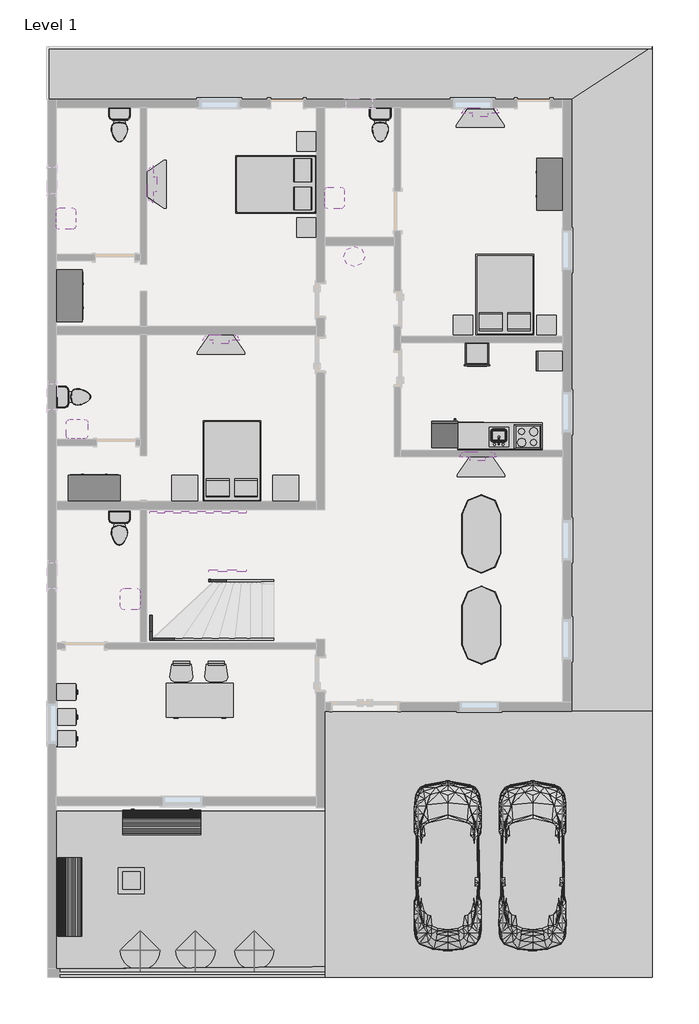
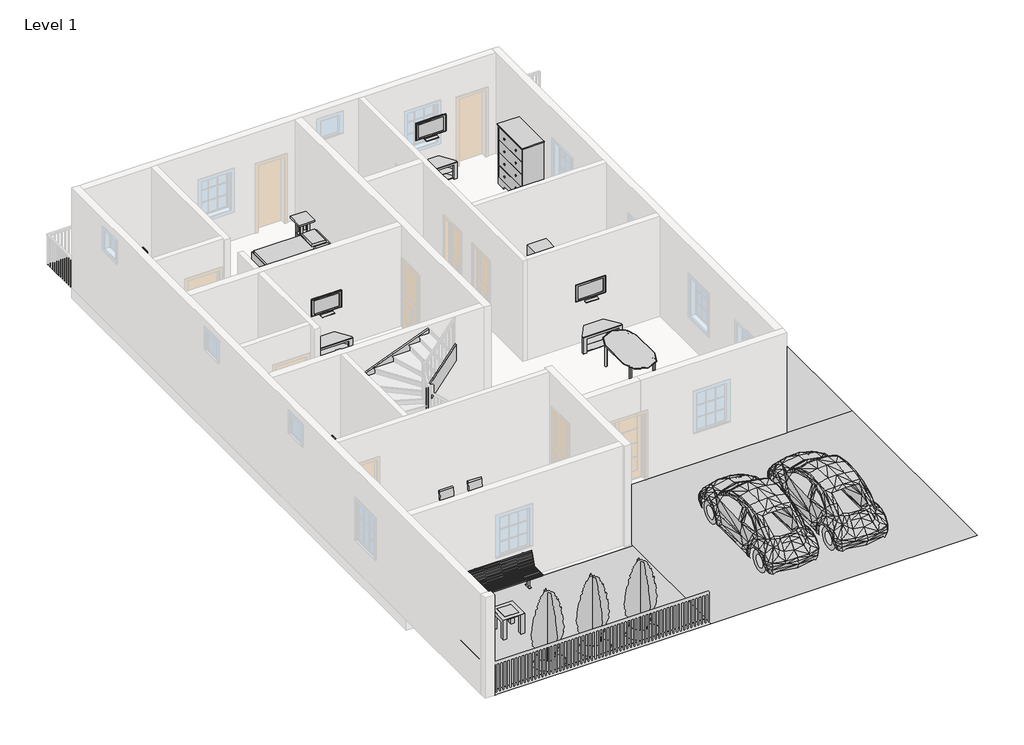
# One storey, part 4 of 4: 30 furniture elements, 13 proxies, 10 flow terminals, 8 members, 5 geographic elements.
"""IFC4 building model written with IfcOpenShell, lengths in millimetres."""

from ifc_helpers import new_model, si_unit, frame, origin, place, context, project, spatial, polyline, outline, extrude, triangles, transform, mapped, element, save
from components import proxy_7e1014cc, proxy_a6faaae8, proxy_45b28599, kitchenette_medium_kitchenette_medium_844211aa, proxy_8b8c2dc4, rpc_beetle_rpc_beetle_3ce7ba48, proxy_c523a7b7, flow_terminal_871c2e40, flow_terminal_d49f872f, flow_terminal_62a433f7, toilet_domestic_3d_toilet_domestic_3d_f7549cf7, toilet_domestic_3d_toilet_domestic_3d_183bbd19, furniture_c8abb964, furniture_bb55ed6b, chair_desk_chair_desk_ccc35c8f, furniture_c6510c7c, furniture_013ab306, furniture_9fa109b2, furniture_56245f3a, tv_stand_tv_stand_6ce107e5, furniture_b5c51a22, furniture_2c34a4f9, furniture_097b63cf, furniture_5bc9ed15, geographic_element_235d1464, rpc_tree_conifer_0001_chinese_juniper_7_1b9786cd

model = new_model("IFC4")

# Units and contexts
model_context = context("Model", 3, world=origin())
ifc_project = project(units=[si_unit("LENGTHUNIT", "METRE", prefix="MILLI")], contexts=[model_context])

# Site, building, storey
site = spatial("IfcSite", under=ifc_project)
building = spatial("IfcBuilding", under=site)
storey = spatial("IfcBuildingStorey", under=building, Name="Level 1", Elevation=0.0)

# Proxies
placement = place(None, origin())
element("IfcBuildingElementProxy", 1, Name="Building Element Proxy", at=placement, inside=storey, context=model_context, shape_type="Tessellation", body=[
    triangles([(-5541.2013062, 9210.7988297, 0.0), (-5541.2013062, 10429.9982483, 0.0), (8581.1988876, 10429.9982483, 0.0), (6701.5985001, 9210.7988297, 0.0)], [[2, 1, 4], [4, 3, 2]], closed=False),
])
element("IfcBuildingElementProxy", 2, Name="Building Element Proxy", at=placement, inside=storey, context=model_context, shape_type="Tessellation", body=[
    triangles([(6701.5985001, 9210.7988297, 0.0), (8581.1988876, 10429.9982483, 0.0), (6701.5985001, -5089.4009766, 0.0), (8581.1988876, -5089.4009766, 0.0)], [[1, 3, 4], [4, 2, 1]], closed=False),
])
element("IfcBuildingElementProxy", 3, Name="Building Element Proxy", at=placement, inside=storey, context=model_context, shape_type="Tessellation", body=[
    triangles([(935.7986212, -11312.4013641, 0.0), (935.7986212, -7350.0013641, 0.0), (935.7986212, -5089.4009766, 0.0), (8581.1988876, -5089.4009766, 0.0), (8581.1988876, -11312.4013641, 0.0)], [[2, 4, 3], [2, 5, 4], [5, 2, 1]], closed=False),
])
element("IfcBuildingElementProxy", 4, Name="Building Element Proxy", at=placement, inside=storey, context=model_context, shape_type="Tessellation", body=[
    triangles([(-5338.0014999, -11109.2009766, 0.0), (-5329.5107391, -7423.5707108, 0.0), (934.8501326, -7422.4108978, 0.0), (935.7986212, -11058.4017517, 0.0)], [[2, 1, 4], [4, 3, 2]], closed=False),
])
element("IfcBuildingElementProxy", 5, Name="Building Element Proxy", at=placement, inside=storey, context=model_context, shape_type="Tessellation", body=[
    triangles([(932.4697546, -11067.6383972, 0.0), (935.7986212, -11312.4013641, 0.0), (-5261.8014999, -11109.2009766, 0.0), (-5242.6887131, -11312.4013641, 0.0), (-5261.8014999, -11312.4013641, 0.0)], [[3, 5, 4], [4, 2, 1], [4, 1, 3]], closed=False),
])
proxy_shape = proxy_7e1014cc(model_context)
element("IfcBuildingElementProxy", 6, Name="18\" x 24\" x 34 1/2\"", ObjectType="18\" x 24\" x 34 1/2\"", at=placement, inside=storey, context=model_context, shape_type="MappedRepresentation", body=[
    mapped(proxy_shape, transform((5927.1490822, 3395.5162793, 0.0), x_axis=(0.0, -1.0000000000000009, 0.0), y_axis=(1.0000000000000009, 0.0, 0.0), z_axis=(0.0, 0.0, 1.0))),
])
proxy_2_shape = proxy_a6faaae8(model_context)
element("IfcBuildingElementProxy", 7, Name="Cook Top-4 Unit2 : 22\" x 20\"", ObjectType="Cook Top-4 Unit2 : 22\" x 20\"", at=placement, inside=storey, context=model_context, shape_type="MappedRepresentation", body=[
    mapped(proxy_2_shape, transform((5672.898647, 1311.3988108, 0.0), x_axis=(-1.0000000000000004, 0.0, 0.0), y_axis=(0.0, -1.0000000000000004, 0.0), z_axis=(0.0, 0.0, 1.0))),
])
proxy_3_shape = proxy_45b28599(model_context)
element("IfcBuildingElementProxy", 8, Name="Dishwasher : 24\" x 24\" x 34\"", ObjectType="Dishwasher : 24\" x 24\" x 34\"", at=placement, inside=storey, context=model_context, shape_type="MappedRepresentation", body=[
    mapped(proxy_3_shape, transform((4721.7161155, 1603.2483756, 0.0), x_axis=(-1.0000000000000004, 0.0, 0.0), y_axis=(0.0, -1.0000000000000004, 0.0), z_axis=(0.0, 0.0, 1.0))),
])
kitchenette_medium_kitchenette_medium_shape = kitchenette_medium_kitchenette_medium_844211aa(model_context)
element("IfcBuildingElementProxy", 9, Name="Kitchenette - Medium : Kitchenette - Medium", ObjectType="Kitchenette - Medium : Kitchenette - Medium", at=placement, inside=storey, context=model_context, shape_type="MappedRepresentation", body=[
    mapped(kitchenette_medium_kitchenette_medium_shape, transform((5348.7363519, 1006.5988108, 0.0), x_axis=(-1.0000000000000004, 0.0, 0.0), y_axis=(0.0, -1.0000000000000004, 0.0), z_axis=(0.0, 0.0, 1.0))),
])
proxy_4_shape = proxy_8b8c2dc4(model_context)
element("IfcBuildingElementProxy", 10, Name="Oven Double-Built-in : 21 1/2\" x 39 1/4\" x 21\"", ObjectType="Oven Double-Built-in : 21 1/2\" x 39 1/4\" x 21\"", at=placement, inside=storey, context=model_context, shape_type="MappedRepresentation", body=[
    mapped(proxy_4_shape, transform((4526.9735743, 3126.1329519, 0.0), x_axis=(1.0, 0.0, 0.0), y_axis=(0.0, 1.0, 0.0), z_axis=(0.0, 0.0, 1.0))),
])
rpc_beetle_rpc_beetle_shape = rpc_beetle_rpc_beetle_3ce7ba48(model_context)
element("IfcBuildingElementProxy", 11, Name="RPC Beetle : RPC Beetle", ObjectType="RPC Beetle : RPC Beetle", at=placement, inside=storey, context=model_context, shape_type="MappedRepresentation", body=[
    mapped(rpc_beetle_rpc_beetle_shape, transform((5787.198647, -9940.8011892, 0.0), x_axis=(1.0, 0.0, 0.0), y_axis=(0.0, 1.0, 0.0), z_axis=(0.0, 0.0, 1.0))),
])
element("IfcBuildingElementProxy", 12, Name="RPC Beetle : RPC Beetle", ObjectType="RPC Beetle : RPC Beetle", at=placement, inside=storey, context=model_context, shape_type="MappedRepresentation", body=[
    mapped(rpc_beetle_rpc_beetle_shape, transform((3805.998647, -9940.8011892, 0.0), x_axis=(1.0, 0.0, 0.0), y_axis=(0.0, 1.0, 0.0), z_axis=(0.0, 0.0, 1.0))),
])
proxy_5_shape = proxy_c523a7b7(model_context)
element("IfcBuildingElementProxy", 13, Name="Refrigerator : 24\" x 25\" LH", ObjectType="Refrigerator : 24\" x 25\" LH", at=placement, inside=storey, context=model_context, shape_type="MappedRepresentation", body=[
    mapped(proxy_5_shape, transform((3736.148647, 1357.0477823, 0.0), x_axis=(-1.0000000000000004, 0.0, 0.0), y_axis=(0.0, -1.0000000000000004, 0.0), z_axis=(0.0, 0.0, 1.0))),
])

# Flow terminals
flow_terminal_shape = flow_terminal_871c2e40(model_context)
element("IfcFlowTerminal", 14, ObjectType="Sink Kitchen-Island : 18\" x 18\"", at=placement, inside=storey, context=model_context, shape_type="MappedRepresentation", body=[
    mapped(flow_terminal_shape, transform((5015.4878876, 1313.7442119, -14.4), x_axis=(-1.0000000000000004, 0.0, 0.0), y_axis=(0.0, -1.0000000000000004, 0.0), z_axis=(0.0, 0.0, 1.0))),
])
flow_terminal_2_shape = flow_terminal_d49f872f(model_context)
element("IfcFlowTerminal", 15, ObjectType="Sink Vanity-Round : 19\" x 19\"", at=placement, inside=storey, context=model_context, shape_type="MappedRepresentation", body=[
    mapped(flow_terminal_2_shape, transform((1524.9469064, 5444.8120813, 914.4), x_axis=(1.0, 0.0, 0.0), y_axis=(0.0, 1.0, 0.0), z_axis=(0.0, 0.0, 1.0))),
])
flow_terminal_3_shape = flow_terminal_62a433f7(model_context)
element("IfcFlowTerminal", 16, ObjectType="Sink Vanity-Square : 20\" x 18\"", at=placement, inside=storey, context=model_context, shape_type="MappedRepresentation", body=[
    mapped(flow_terminal_3_shape, transform((-5157.8559519, 6401.1095702, 914.4), x_axis=(0.0, 1.0, 0.0), y_axis=(-1.0, 0.0, 0.0), z_axis=(0.0, 0.0, 1.0))),
])
element("IfcFlowTerminal", 17, ObjectType="Sink Vanity-Square : 20\" x 18\"", at=placement, inside=storey, context=model_context, shape_type="MappedRepresentation", body=[
    mapped(flow_terminal_3_shape, transform((1115.9440481, 6883.7095702, 914.4), x_axis=(0.0, 1.0000000000000002, 0.0), y_axis=(-1.0000000000000002, 0.0, 0.0), z_axis=(0.0, 0.0, 1.0))),
])
element("IfcFlowTerminal", 18, ObjectType="Sink Vanity-Square : 20\" x 18\"", at=placement, inside=storey, context=model_context, shape_type="MappedRepresentation", body=[
    mapped(flow_terminal_3_shape, transform((-4839.7121124, 1453.4442119, 914.4), x_axis=(-1.0, 0.0, 0.0), y_axis=(0.0, -1.0, 0.0), z_axis=(0.0, 0.0, 1.0))),
])
element("IfcFlowTerminal", 19, ObjectType="Sink Vanity-Square : 20\" x 18\"", at=placement, inside=storey, context=model_context, shape_type="MappedRepresentation", body=[
    mapped(flow_terminal_3_shape, transform((-3562.3467541, -2457.5119486, 914.4), x_axis=(0.0, -1.0000000000000004, 0.0), y_axis=(1.0000000000000004, 0.0, 0.0), z_axis=(0.0, 0.0, 1.0))),
])
toilet_domestic_3d_toilet_domestic_3d_shape = toilet_domestic_3d_toilet_domestic_3d_f7549cf7(model_context)
toilet_domestic_3d_toilet_domestic_3d_2_shape = toilet_domestic_3d_toilet_domestic_3d_183bbd19(model_context)
element("IfcFlowTerminal", 20, ObjectType="Toilet-Domestic-3D : Toilet-Domestic-3D", at=placement, inside=storey, context=model_context, shape_type="MappedRepresentation", body=[
    mapped(toilet_domestic_3d_toilet_domestic_3d_shape, transform((-4843.3053257, 2251.1988108, 0.0), x_axis=(0.0, 1.0000000000000002, 0.0), y_axis=(-1.0000000000000002, 0.0, 0.0), z_axis=(0.0, 0.0, 1.0))),
    mapped(toilet_domestic_3d_toilet_domestic_3d_2_shape, transform((-4843.3053257, 2251.1988108, 0.0), x_axis=(0.0, 1.0000000000000002, 0.0), y_axis=(-1.0000000000000002, 0.0, 0.0), z_axis=(0.0, 0.0, 1.0))),
])
element("IfcFlowTerminal", 21, ObjectType="Toilet-Domestic-3D : Toilet-Domestic-3D", at=placement, inside=storey, context=model_context, shape_type="MappedRepresentation", body=[
    mapped(toilet_domestic_3d_toilet_domestic_3d_shape, transform((-3864.801353, 8512.9027835, 0.0), x_axis=(1.0, 0.0, 0.0), y_axis=(0.0, 1.0, 0.0), z_axis=(0.0, 0.0, 1.0))),
    mapped(toilet_domestic_3d_toilet_domestic_3d_2_shape, transform((-3864.801353, 8512.9027835, 0.0), x_axis=(1.0, 0.0, 0.0), y_axis=(0.0, 1.0, 0.0), z_axis=(0.0, 0.0, 1.0))),
])
element("IfcFlowTerminal", 22, ObjectType="Toilet-Domestic-3D : Toilet-Domestic-3D", at=placement, inside=storey, context=model_context, shape_type="MappedRepresentation", body=[
    mapped(toilet_domestic_3d_toilet_domestic_3d_shape, transform((2231.198647, 8512.9027835, 0.0), x_axis=(1.0, 0.0, 0.0), y_axis=(0.0, 1.0, 0.0), z_axis=(0.0, 0.0, 1.0))),
    mapped(toilet_domestic_3d_toilet_domestic_3d_2_shape, transform((2231.198647, 8512.9027835, 0.0), x_axis=(1.0, 0.0, 0.0), y_axis=(0.0, 1.0, 0.0), z_axis=(0.0, 0.0, 1.0))),
])
element("IfcFlowTerminal", 23, ObjectType="Toilet-Domestic-3D : Toilet-Domestic-3D", at=placement, inside=storey, context=model_context, shape_type="MappedRepresentation", body=[
    mapped(toilet_domestic_3d_toilet_domestic_3d_shape, transform((-3864.801353, -910.4972165, 0.0), x_axis=(1.0, 0.0, 0.0), y_axis=(0.0, 1.0, 0.0), z_axis=(0.0, 0.0, 1.0))),
    mapped(toilet_domestic_3d_toilet_domestic_3d_2_shape, transform((-3864.801353, -910.4972165, 0.0), x_axis=(1.0, 0.0, 0.0), y_axis=(0.0, 1.0, 0.0), z_axis=(0.0, 0.0, 1.0))),
])

# Furniture
furniture_shape = furniture_c8abb964(model_context)
element("IfcFurniture", 24, ObjectType="Bed-Box : Double 53\" x 74\"", at=placement, inside=storey, context=model_context, shape_type="MappedRepresentation", body=[
    mapped(furniture_shape, transform((-896.748894, 518.1693026, 0.0), x_axis=(-1.0, 0.0, 0.0), y_axis=(0.0, -1.0, 0.0), z_axis=(0.0, 0.0, 1.0))),
])
element("IfcFurniture", 25, ObjectType="Bed-Box : Double 53\" x 74\"", at=placement, inside=storey, context=model_context, shape_type="MappedRepresentation", body=[
    mapped(furniture_shape, transform((27.2281552, 7556.0512698, 0.0), x_axis=(0.0, -1.0000000000000002, 0.0), y_axis=(1.0000000000000002, 0.0, 0.0), z_axis=(0.0, 0.0, 1.0))),
])
element("IfcFurniture", 26, ObjectType="Bed-Box : Double 53\" x 74\"", at=placement, inside=storey, context=model_context, shape_type="MappedRepresentation", body=[
    mapped(furniture_shape, transform((5478.651106, 4404.3693026, 0.0), x_axis=(-1.0, 0.0, 0.0), y_axis=(0.0, -1.0, 0.0), z_axis=(0.0, 0.0, 1.0))),
])
furniture_2_shape = furniture_bb55ed6b(model_context)
element("IfcFurniture", 27, ObjectType="Cabinet-File 2 Drawer : 15\" x 18\"", at=placement, inside=storey, context=model_context, shape_type="MappedRepresentation", body=[
    mapped(furniture_2_shape, transform((-5251.5356531, -5609.2047422, 0.0), x_axis=(0.0, 1.0000000000000002, 0.0), y_axis=(-1.0000000000000002, 0.0, 0.0), z_axis=(0.0, 0.0, 1.0))),
])
element("IfcFurniture", 28, ObjectType="Cabinet-File 2 Drawer : 15\" x 18\"", at=placement, inside=storey, context=model_context, shape_type="MappedRepresentation", body=[
    mapped(furniture_2_shape, transform((-5251.5356531, -5101.2047422, 0.0), x_axis=(0.0, 1.0000000000000002, 0.0), y_axis=(-1.0000000000000002, 0.0, 0.0), z_axis=(0.0, 0.0, 1.0))),
])
element("IfcFurniture", 29, ObjectType="Cabinet-File 2 Drawer : 15\" x 18\"", at=placement, inside=storey, context=model_context, shape_type="MappedRepresentation", body=[
    mapped(furniture_2_shape, transform((-5251.5356531, -4517.0047422, 0.0), x_axis=(0.0, 1.0000000000000002, 0.0), y_axis=(-1.0000000000000002, 0.0, 0.0), z_axis=(0.0, 0.0, 1.0))),
])
chair_desk_chair_desk_shape = chair_desk_chair_desk_ccc35c8f(model_context)
element("IfcFurniture", 30, ObjectType="Chair-Desk : Chair-Desk", at=placement, inside=storey, context=model_context, shape_type="MappedRepresentation", body=[
    mapped(chair_desk_chair_desk_shape, transform((-2417.001353, -3997.2011892, 0.0), x_axis=(-1.0000000000000004, 0.0, 0.0), y_axis=(0.0, -1.0000000000000004, 0.0), z_axis=(0.0, 0.0, 1.0))),
])
element("IfcFurniture", 31, ObjectType="Chair-Desk : Chair-Desk", at=placement, inside=storey, context=model_context, shape_type="MappedRepresentation", body=[
    mapped(chair_desk_chair_desk_shape, transform((-1604.201353, -3997.2011892, 0.0), x_axis=(-1.0000000000000009, 0.0, 0.0), y_axis=(0.0, -1.0000000000000009, 0.0), z_axis=(0.0, 0.0, 1.0))),
])
furniture_3_shape = furniture_c6510c7c(model_context)
element("IfcFurniture", 32, ObjectType="Counter Top w Sink Hole : 24\" Depth", at=placement, inside=storey, context=model_context, shape_type="MappedRepresentation", body=[
    mapped(furniture_3_shape, transform((4815.3363519, 1006.5988108, -14.4), x_axis=(-1.0000000000000004, 0.0, 0.0), y_axis=(0.0, -1.0000000000000004, 0.0), z_axis=(0.0, 0.0, 1.0))),
])
furniture_4_shape = furniture_013ab306(model_context)
element("IfcFurniture", 33, ObjectType="Desk : 60\" x 30\" Student", at=placement, inside=storey, context=model_context, shape_type="MappedRepresentation", body=[
    mapped(furniture_4_shape, transform((-2747.201353, -5216.4011892, 0.0), x_axis=(1.0, 0.0, 0.0), y_axis=(0.0, 1.0, 0.0), z_axis=(0.0, 0.0, 1.0))),
])
furniture_5_shape = furniture_9fa109b2(model_context)
element("IfcFurniture", 34, ObjectType="Dresser : 48\" x 72\" x 24\"", at=placement, inside=storey, context=model_context, shape_type="MappedRepresentation", body=[
    mapped(furniture_5_shape, transform((6556.7616011, 6947.705551, 0.0), x_axis=(0.0, -1.0000000000000007, 0.0), y_axis=(1.0000000000000007, 0.0, 0.0), z_axis=(0.0, 0.0, 1.0))),
])
element("IfcFurniture", 35, ObjectType="Dresser : 48\" x 72\" x 24\"", at=placement, inside=storey, context=model_context, shape_type="MappedRepresentation", body=[
    mapped(furniture_5_shape, transform((-4718.1946128, -245.5641433, 0.0), x_axis=(-1.0000000000000004, 0.0, 0.0), y_axis=(0.0, -1.0000000000000004, 0.0), z_axis=(0.0, 0.0, 1.0))),
])
element("IfcFurniture", 36, ObjectType="Dresser : 48\" x 72\" x 24\"", at=placement, inside=storey, context=model_context, shape_type="MappedRepresentation", body=[
    mapped(furniture_5_shape, transform((-5396.3643071, 4882.5920706, 0.0), x_axis=(0.0, 1.0000000000000002, 0.0), y_axis=(-1.0000000000000002, 0.0, 0.0), z_axis=(0.0, 0.0, 1.0))),
])
furniture_6_shape = furniture_56245f3a(model_context)
element("IfcFurniture", 37, ObjectType="TV - Flat Screen : 32\"", at=placement, inside=storey, context=model_context, shape_type="MappedRepresentation", body=[
    mapped(furniture_6_shape, transform((4571.9431611, 8949.0601872, 1219.2), x_axis=(1.0, 0.0, 0.0), y_axis=(0.0, 1.0, 0.0), z_axis=(0.0, 0.0, 1.0))),
])
element("IfcFurniture", 38, ObjectType="TV - Flat Screen : 32\"", at=placement, inside=storey, context=model_context, shape_type="MappedRepresentation", body=[
    mapped(furniture_6_shape, transform((-3141.3848657, 7220.843325, 1219.2), x_axis=(0.0, 1.0, 0.0), y_axis=(-1.0, 0.0, 0.0), z_axis=(0.0, 0.0, 1.0))),
])
element("IfcFurniture", 39, ObjectType="TV - Flat Screen : 32\"", at=placement, inside=storey, context=model_context, shape_type="MappedRepresentation", body=[
    mapped(furniture_6_shape, transform((-1485.9568389, 3640.4601872, 1219.2), x_axis=(1.0, 0.0, 0.0), y_axis=(0.0, 1.0, 0.0), z_axis=(0.0, 0.0, 1.0))),
])
element("IfcFurniture", 40, ObjectType="TV - Flat Screen : 32\"", at=placement, inside=storey, context=model_context, shape_type="MappedRepresentation", body=[
    mapped(furniture_6_shape, transform((4511.6355628, 914.049371, 1219.2), x_axis=(1.0, 0.0, 0.0), y_axis=(0.0, 1.0, 0.0), z_axis=(0.0, 0.0, 1.0))),
])
tv_stand_tv_stand_shape = tv_stand_tv_stand_6ce107e5(model_context)
element("IfcFurniture", 41, ObjectType="TV Stand : TV Stand", at=placement, inside=storey, context=model_context, shape_type="MappedRepresentation", body=[
    mapped(tv_stand_tv_stand_shape, transform((4442.8106449, 9007.5988108, 0.0), x_axis=(1.0, 0.0, 0.0), y_axis=(0.0, 1.0, 0.0), z_axis=(0.0, 0.0, 1.0))),
])
element("IfcFurniture", 42, ObjectType="TV Stand : TV Stand", at=placement, inside=storey, context=model_context, shape_type="MappedRepresentation", body=[
    mapped(tv_stand_tv_stand_shape, transform((-3229.801353, 7091.7108087, 0.0), x_axis=(0.0, 1.0000000000000002, 0.0), y_axis=(-1.0000000000000002, 0.0, 0.0), z_axis=(0.0, 0.0, 1.0))),
])
element("IfcFurniture", 43, ObjectType="TV Stand : TV Stand", at=placement, inside=storey, context=model_context, shape_type="MappedRepresentation", body=[
    mapped(tv_stand_tv_stand_shape, transform((-1615.0893551, 3698.9988108, 0.0), x_axis=(1.0000000000000007, 0.0, 0.0), y_axis=(0.0, 1.0000000000000007, 0.0), z_axis=(0.0, 0.0, 1.0))),
])
element("IfcFurniture", 44, ObjectType="TV Stand : TV Stand", at=placement, inside=storey, context=model_context, shape_type="MappedRepresentation", body=[
    mapped(tv_stand_tv_stand_shape, transform((4457.5227393, 838.7879946, 0.0), x_axis=(1.0000000000000007, 0.0, 0.0), y_axis=(0.0, 1.0000000000000007, 0.0), z_axis=(0.0, 0.0, 1.0))),
])
furniture_7_shape = furniture_b5c51a22(model_context)
element("IfcFurniture", 45, ObjectType="Table-Coffee : 24\" x 24\" x 24\"", at=placement, inside=storey, context=model_context, shape_type="MappedRepresentation", body=[
    mapped(furniture_7_shape, transform((-3603.6671197, -9147.012267, 0.0), x_axis=(1.0, 0.0, 0.0), y_axis=(0.0, 1.0, 0.0), z_axis=(0.0, 0.0, 1.0))),
])
furniture_8_shape = furniture_2c34a4f9(model_context)
element("IfcFurniture", 46, ObjectType="Table-Dining Oval : 36\" x 72\"", at=placement, inside=storey, context=model_context, shape_type="MappedRepresentation", body=[
    mapped(furniture_8_shape, transform((4235.3002863, -547.3815171, 0.0), x_axis=(0.0, 1.0, 0.0), y_axis=(-1.0, 0.0, 0.0), z_axis=(0.0, 0.0, 1.0))),
])
element("IfcFurniture", 47, ObjectType="Table-Dining Oval : 36\" x 72\"", at=placement, inside=storey, context=model_context, shape_type="MappedRepresentation", body=[
    mapped(furniture_8_shape, transform((4951.4970076, -3484.6208613, 0.0), x_axis=(0.0, -1.0, 0.0), y_axis=(1.0, 0.0, 0.0), z_axis=(0.0, 0.0, 1.0))),
])
furniture_9_shape = furniture_097b63cf(model_context)
element("IfcFurniture", 48, ObjectType="Table-Night Stand : 18\" x 18\" x 24\"", at=placement, inside=storey, context=model_context, shape_type="MappedRepresentation", body=[
    mapped(furniture_9_shape, transform((5885.0650167, 3698.9988108, 0.0), x_axis=(1.0, 0.0, 0.0), y_axis=(0.0, 1.0, 0.0), z_axis=(0.0, 0.0, 1.0))),
])
element("IfcFurniture", 49, ObjectType="Table-Night Stand : 18\" x 18\" x 24\"", at=placement, inside=storey, context=model_context, shape_type="MappedRepresentation", body=[
    mapped(furniture_9_shape, transform((3929.2650167, 3698.9988108, 0.0), x_axis=(1.0, 0.0, 0.0), y_axis=(0.0, 1.0, 0.0), z_axis=(0.0, 0.0, 1.0))),
])
element("IfcFurniture", 50, ObjectType="Table-Night Stand : 18\" x 18\" x 24\"", at=placement, inside=storey, context=model_context, shape_type="MappedRepresentation", body=[
    mapped(furniture_9_shape, transform((271.6650167, 5984.9988108, 0.0), x_axis=(1.0, 0.0, 0.0), y_axis=(0.0, 1.0, 0.0), z_axis=(0.0, 0.0, 1.0))),
])
element("IfcFurniture", 51, ObjectType="Table-Night Stand : 18\" x 18\" x 24\"", at=placement, inside=storey, context=model_context, shape_type="MappedRepresentation", body=[
    mapped(furniture_9_shape, transform((271.6650167, 7991.5988108, 0.0), x_axis=(1.0, 0.0, 0.0), y_axis=(0.0, 1.0, 0.0), z_axis=(0.0, 0.0, 1.0))),
])
furniture_10_shape = furniture_5bc9ed15(model_context)
element("IfcFurniture", 52, ObjectType="Table-Night Stand : 24\" x 24\" x 30\"", at=placement, inside=storey, context=model_context, shape_type="MappedRepresentation", body=[
    mapped(furniture_10_shape, transform((-287.1349833, -187.2011892, 0.0), x_axis=(1.0, 0.0, 0.0), y_axis=(0.0, 1.0, 0.0), z_axis=(0.0, 0.0, 1.0))),
])
element("IfcFurniture", 53, ObjectType="Table-Night Stand : 24\" x 24\" x 30\"", at=placement, inside=storey, context=model_context, shape_type="MappedRepresentation", body=[
    mapped(furniture_10_shape, transform((-2649.3349833, -187.2011892, 0.0), x_axis=(1.0, 0.0, 0.0), y_axis=(0.0, 1.0, 0.0), z_axis=(0.0, 0.0, 1.0))),
])

# Geographic elements
geographic_element_shape = geographic_element_235d1464(model_context)
element("IfcGeographicElement", 54, ObjectType="Park Bench : 72\"", at=placement, inside=storey, context=model_context, shape_type="MappedRepresentation", body=[
    mapped(geographic_element_shape, transform((-5058.601353, -9432.8011892, 0.0), x_axis=(0.0, 1.0000000000000002, 0.0), y_axis=(-1.0000000000000002, 0.0, 0.0), z_axis=(0.0, 0.0, 1.0))),
])
element("IfcGeographicElement", 55, ObjectType="Park Bench : 72\"", at=placement, inside=storey, context=model_context, shape_type="MappedRepresentation", body=[
    mapped(geographic_element_shape, transform((-2874.201353, -7654.8011892, 0.0), x_axis=(1.0000000000000007, 0.0, 0.0), y_axis=(0.0, 1.0000000000000007, 0.0), z_axis=(0.0, 0.0, 1.0))),
])
rpc_tree_conifer_0001_chinese_juniper_7_shape = rpc_tree_conifer_0001_chinese_juniper_7_1b9786cd(model_context)
element("IfcGeographicElement", 56, ObjectType="RPC Tree - Conifer.0001 : Chinese Juniper - 7'", at=placement, inside=storey, context=model_context, shape_type="MappedRepresentation", body=[
    mapped(rpc_tree_conifer_0001_chinese_juniper_7_shape, transform((-3382.3980241, -10677.4011892, 0.0), x_axis=(1.0, 0.0, 0.0), y_axis=(0.0, 1.0, 0.0), z_axis=(0.0, 0.0, 1.0))),
])
element("IfcGeographicElement", 57, ObjectType="RPC Tree - Conifer.0001 : Chinese Juniper - 7'", at=placement, inside=storey, context=model_context, shape_type="MappedRepresentation", body=[
    mapped(rpc_tree_conifer_0001_chinese_juniper_7_shape, transform((-2086.9980241, -10677.4011892, 0.0), x_axis=(1.0, 0.0, 0.0), y_axis=(0.0, 1.0, 0.0), z_axis=(0.0, 0.0, 1.0))),
])
element("IfcGeographicElement", 58, ObjectType="RPC Tree - Conifer.0001 : Chinese Juniper - 7'", at=placement, inside=storey, context=model_context, shape_type="MappedRepresentation", body=[
    mapped(rpc_tree_conifer_0001_chinese_juniper_7_shape, transform((-715.3980241, -10677.4011892, 0.0), x_axis=(1.0, 0.0, 0.0), y_axis=(0.0, 1.0, 0.0), z_axis=(0.0, 0.0, 1.0))),
])

# Members
element("IfcMember", 59, ObjectType="Stringer - 2\" Width", at=placement, inside=storey, context=model_context, shape_type="SweptSolid", body=[
    extrude(outline(polyline([(0.0, -254.2696611), (252.5395012, -254.2696611), (1410.2864637, -3102.801353), (1081.2731753, -3102.801353), (0.0, -442.4264981), (0.0, -254.2696611)])), frame((0.0, -3438.4011892, 0.0), z_axis=(0.0, 1.0, 0.0), x_axis=(0.0, 0.0, 1.0)), (0.0, 0.0, 1.0), 50.8),
])
element("IfcMember", 60, ObjectType="Stringer - 2\" Width", at=placement, inside=storey, context=model_context, shape_type="SweptSolid", body=[
    extrude(outline(polyline([(-3102.801353, -3438.4011892), (-3153.601353, -3438.4011892), (-3153.601353, -3233.5988119), (-3102.801353, -3233.5988119), (-3102.801353, -3438.4011892)])), frame((0.0, 0.0, 1081.2731753), z_axis=(0.0, 0.0, 1.0), x_axis=(1.0, 0.0, 0.0)), (0.0, 0.0, 1.0), 329.0132884),
])
element("IfcMember", 61, ObjectType="Stringer - 2\" Width", at=placement, inside=storey, context=model_context, shape_type="SweptSolid", body=[
    extrude(outline(polyline([(-3233.5988119, 1081.2731753), (-3233.5988119, 1410.2864637), (-482.1324236, 2261.4341506), (-466.6011892, 2261.4341506), (-466.6011892, 1937.2253455), (-3233.5988119, 1081.2731753)])), frame((-3153.601353, 0.0, 0.0), z_axis=(1.0, 0.0, 0.0), x_axis=(0.0, 1.0, 0.0)), (0.0, 0.0, 1.0), 50.8),
])
element("IfcMember", 62, ObjectType="Stringer - 2\" Width", at=placement, inside=storey, context=model_context, shape_type="SweptSolid", body=[
    extrude(outline(polyline([(-3153.601353, -466.6011892), (-3153.601353, -415.8011892), (-2802.5254205, -415.8011892), (-2802.5254205, -466.6011892), (-3153.601353, -466.6011892)])), frame((0.0, 0.0, 1942.3836276), z_axis=(0.0, 0.0, 1.0), x_axis=(1.0, 0.0, 0.0)), (0.0, 0.0, 1.0), 319.050523),
])
element("IfcMember", 63, ObjectType="Stringer - 2\" Width", at=placement, inside=storey, context=model_context, shape_type="SweptSolid", body=[
    extrude(outline(polyline([(2261.4341506, -2802.5254205), (1942.3836276, -2802.5254205), (2692.3099341, -898.8739925), (3011.3604571, -898.8739925), (2261.4341506, -2802.5254205)])), frame((0.0, -466.6011892, 0.0), z_axis=(0.0, 1.0, 0.0), x_axis=(0.0, 0.0, 1.0)), (0.0, 0.0, 1.0), 50.8),
])
element("IfcMember", 64, ObjectType="Stringer - 2\" Width", at=placement, inside=storey, context=model_context, shape_type="SweptSolid", body=[
    extrude(outline(polyline([(0.0, -254.2696611), (158.2306385, -254.2696611), (1536.3658755, -1731.201353), (1119.4814104, -1731.201353), (0.0, -531.4659939), (0.0, -254.2696611)])), frame((0.0, -2066.8011892, 0.0), z_axis=(0.0, 1.0, 0.0), x_axis=(0.0, 0.0, 1.0)), (0.0, 0.0, 1.0), 50.8),
])
element("IfcMember", 65, ObjectType="Stringer - 2\" Width", at=placement, inside=storey, context=model_context, shape_type="SweptSolid", body=[
    extrude(outline(polyline([(-2066.8011892, 1166.8832438), (-2066.8011892, 1798.0484781), (-1862.3747573, 2231.9720128), (-1838.2011892, 2231.9720128), (-1838.2011892, 1568.1008109), (-2027.2194588, 1166.8832438), (-2066.8011892, 1166.8832438)])), frame((-1782.001353, 0.0, 0.0), z_axis=(1.0, 0.0, 0.0), x_axis=(0.0, 1.0, 0.0)), (0.0, 0.0, 1.0), 50.8),
])
element("IfcMember", 66, ObjectType="Stringer - 2\" Width", at=placement, inside=storey, context=model_context, shape_type="SweptSolid", body=[
    extrude(outline(polyline([(2231.9720128, -1782.001353), (1734.1247026, -1782.001353), (2874.6439848, -898.8739925), (3372.491295, -898.8739925), (2231.9720128, -1782.001353)])), frame((0.0, -1838.2011892, 0.0), z_axis=(0.0, 1.0, 0.0), x_axis=(0.0, 0.0, 1.0)), (0.0, 0.0, 1.0), 50.8),
])

save(model, "model.ifc")

# Revit data of these elements
# Type "18\" x 24\" x 34 1/2\""
#   Label = "T"
#   Assembly Code = "E1090400"
#   Depth = 2' - 0"
#   Height = 2' - 10 1/2"
#   Width = 1' - 6"
#   Panel Face Material = Plastic, Opaque Black
#   Trach Compact. Material = Steel, Paint Finish, Ivory, Matte
#   Default Elevation = 0
# Type "Cook Top-4 Unit2 : 22\" x 20\""
#   Depth = 1' - 8"
#   Width = 1' - 10"
#   Burner Material = Steel, Chrome Plated
#   Cooktop Material = Steel, Polished
#   Default Elevation = 0
#   Assembly Code = ""
# Type "Dishwasher : 24\" x 24\" x 34\""
#   Label = "DW"
#   Assembly Code = "E1090400"
#   Depth = 2' - 0"
#   Height = 2' - 10"
#   Width = 2' - 0"
#   Dishwasher Material = Steel, Paint Finish, Ivory, Glossy
#   Panel Face Material = Plastic, Opaque Black
#   Default Elevation = 0
# Type "Kitchenette - Medium : Kitchenette - Medium"
#   Assembly Code = "E1090400"
#   Counter Length = 6' - 6"
#   Cabinet Width = 4' - 6"
#   Cabinet Height = 2' - 10 1/2"
#   Cabinet Depth = 2' - 0"
#   Toe Depth = 0' - 3"
#   Toe Height = 0' - 3 1/2"
#   Cabinet Material = Cabinets
#   Door/Drawer Material = Cabinets
#   Handle Material = Cabinets - Handles
#   Default Elevation = 0
# Type "Oven Double-Built-in : 21 1/2\" x 39 1/4\" x 21\""
#   Label = "OVEN"
#   Assembly Code = "E1090400"
#   Depth = 1' - 9"
#   Height = 3' - 3 1/4"
#   Width = 1' - 9 1/2"
#   Oven Material = Metal - Stainless Steel, Polished
#   Default Elevation = 0
# Type "RPC Beetle : RPC Beetle"
#   built-in parameter 1005195 = "RPC-16-0U6E-L4EG-ENH1-J3KF-SVEL-0TX4-C0"
#   Height = 0
# Type "Refrigerator : 24\" x 25\" LH"
#   Label = "REF."
#   Assembly Code = "E1090400"
#   Depth = 2' - 0 3/4"
#   Handle = 0' - 1 1/2"
#   Height = 5' - 3 1/2"
#   Rear Clearance = 0' - 2"
#   Top Door Height = 1' - 8"
#   Width = 1' - 11 1/2"
#   Material = Steel, Paint Finish, Ivory, Glossy
#   Default Elevation = 0
# Type "Sink Kitchen-Island : 18\" x 18\""
#   Assembly Code = "D2010410"
#   Counter Height = 3' - 0"
#   Depth = 1' - 6"
#   Width = 1' - 6"
#   Faucet Material = Steel, Polished
#   Sink Material = Steel, Polished
#   Default Elevation = 0
# Type "Sink Vanity-Round : 19\" x 19\""
#   Assembly Code = "D2010400"
#   Top Of Counter = 2' - 7"
#   Basin Material = Porcelain, Linen
#   Faucet Material = Steel, Polished
#   Default Elevation = 0
# Type "Sink Vanity-Square : 20\" x 18\""
#   Assembly Code = "D2010400"
#   Counter Height = 2' - 7"
#   Depth = 1' - 6"
#   Width = 1' - 8"
#   Basin Material = Porcelain, Linen
#   Faucet Material = Steel, Polished
#   Default Elevation = 0
# Type "Toilet-Domestic-3D : Toilet-Domestic-3D"
#   Assembly Code = "D2010110"
#   Toilet - Bowl/Basin Material = Porcelain, Linen
#   Toilet - Seat Material = Laminate, Linen, Matte
#   Default Elevation = 0
# Type "Bed-Box : Double 53\" x 74\""
#   Assembly Code = "E2020200"
#   Length = 6' - 2"
#   Width = 4' - 5"
#   Frame Material = Birch
#   Mattress Material = Linen, White
#   Default Elevation = 0
# Type "Cabinet-File 2 Drawer : 15\" x 18\""
#   Assembly Code = "E2020200"
#   Depth = 1' - 6"
#   Height = 2' - 5"
#   Width = 1' - 3"
#   Cabinet Material = Steel, Paint Finish, Ivory, Glossy
#   Handle Material = Steel, Chrome Plated
#   Default Elevation = 0
# Type "Chair-Desk : Chair-Desk"
#   Assembly Code = "E2020200"
#   Seat/Back Material = Textile - Slate Blue
#   Base Material = Steel, Chrome Plated
#   Default Elevation = 0
# Type "Counter Top w Sink Hole : 24\" Depth"
#   Assembly Code = "C1030400"
#   Counter Thickness = 0' - 1 1/2"
#   Depth = 2' - 1"
#   Height = 3' - 0"
#   Length [instance default] = 8' - 0"
#   Sink Location [instance default] = 2' - 0"
#   Sink Location To Wall [instance default] = 0' - 6"
#   Sink Opening Depth [instance default] = 1' - 3"
#   Sink Opening Width [instance default] = 2' - 3"
#   Counter Top Material = none
#   Default Elevation = 0
# Type "Desk : 60\" x 30\" Student"
#   Assembly Code = "E2020200"
#   Depth = 2' - 6"
#   Height = 2' - 6"
#   Leg Height = 0' - 6"
#   Width = 5' - 0"
#   Body Material = Laminate, Ivory, Matte
#   Handle/Leg Material = Steel, Chrome Plated
#   Top Material = Cherry
#   Default Elevation = 0
# Type "Dresser : 48\" x 72\" x 24\""
#   Assembly Code = "E2020200"
#   Depth = 2' - 0"
#   Height = 6' - 0"
#   Width = 4' - 0"
#   Dresser Material = Laminate - Ivory, Glossy
#   Drawer Material = Laminate, Ivory, Matte
#   Knob Material = Cherry
#   Default Elevation = 0
# Type "TV - Flat Screen : 32\""
#   SinAng = 0' - 0.0193"
#   L = 2' - 3.79372"
#   H = 1' - 3.6354"
#   Thickness = 0' - 4.33071"
#   Diagonal = 2' - 7.88976"
#   CosAng = 0' - 0.03431"
#   Stand [instance default] = yes
#   Default Elevation = 0
# Type "TV Stand : TV Stand"
#   Depth = 1' - 6"
#   Width = 3' - 8"
#   Height = 1' - 7 1/2"
#   Finish = Melamine - Gray
#   Default Elevation = 0
# Type "Table-Coffee : 24\" x 24\" x 24\""
#   Assembly Code = "E2020200"
#   Height = 2' - 0"
#   Length = 2' - 0"
#   Width = 2' - 0"
#   Top Material = none
#   Frame Material = none
#   Default Elevation = 0
# Type "Table-Dining Oval : 36\" x 72\""
#   Assembly Code = "E2020200"
#   Length = 6' - 0"
#   Width = 3' - 0"
#   Base Material = Steel, Chrome Plated
#   Top Material = Glass - Clear, Grey
#   Default Elevation = 0
#   Description = (empty or 0)
# Type "Table-Night Stand : 18\" x 18\" x 24\""
#   Assembly Code = "E2020200"
#   Depth = 1' - 6"
#   Height = 2' - 0"
#   Width = 1' - 6"
#   Base Material = Birch
#   Top Material = Laminate, Ivory, Matte
#   Default Elevation = 0
# Type "Table-Night Stand : 24\" x 24\" x 30\""
#   Assembly Code = "E2020200"
#   Depth = 2' - 0"
#   Height = 2' - 6"
#   Width = 2' - 0"
#   Base Material = Birch
#   Top Material = Laminate, Ivory, Matte
#   Default Elevation = 0
# Type "Park Bench : 72\""
#   Length = 6' - 0"
#   Seat Material = Wood - Teak
#   Frame Material = Steel, Paint Finish, Dark Gray, Matte
# Type "RPC Tree - Conifer.0001 : Chinese Juniper - 7'"
#   built-in parameter 1005198 = "{2, 15},{39, RPC-16-FUM3-UUQ0-UBF0-N000-ST1L-LVER-AU},{1, 0},{1, 0},{2, 13},{1, 8},{5, Color},{1, 0},{1, 0},{3, 0.8},{3, 0.8},{3, 0.8},{1, 8},{7, BBoxMin},{1, 0},{1, 0},{1, 0},{1, 0},{1, 0},{1, 8},{7, BBoxMax},{1, 0},{1, 0},{1, 0},{1, 0},{1, 0},{2, 11},{9, RPCTypeId},{1, 0},{1, 0},{39, RPC-16-FUM3-UUQ0-UBF0-N000-ST1L-LVER-AU},{1, 6},{14, RPCPlantHeight},{1, 0},{1, 0},{1, 7},{2, 11},{7, keyword},{1, 0},{1, 0},{34, :RPCs:Trees [General]:Geometry:RPC},{2, 11},{8, category},{1, 0},{1, 0},{15, Trees [General]},{2, 11},{12, LocalizedUID},{1, 0},{1, 0},{15, Chinese Juniper},{2, 14},{6, Height},{1, 0},{1, 0},{1, 7},{1, 2},{16, Cast Reflections},{1, 0},{1, 0},{1, 0},{1, 2},{12, Cast Shadows},{1, 0},{1, 0},{1, 1},{1, 2},{9, Lock View},{1, 0},{1, 0},{1, 0},{1, 4},{5, ViewC},{1, 0},{1, 0},{1, 0},{21, assetlibrary_base.fbx},{1, 5},"
#   built-in parameter 1005195 = "RPC-16-FUM3-UUQ0-UBF0-N000-ST1L-LVER-AU"
#   Type Comments = "Chinese Juniper"
#   Assembly Code = "G2050500"
#   Height = 7' - 0"
#   Description = (empty or 0)
#   Default Elevation = 0
# Elements 1, 2, 3, 4, 5 (IfcBuildingElementProxy)
#   Material = none
#   Phase Created = New Construction
# Element 6 (IfcBuildingElementProxy, "18\" x 24\" x 34 1/2\"")
#   Phase Created = New Construction
#   Materials on its faces: "Steel, Paint Finish, Ivory, Matte", "Plastic, Opaque Black"
# Element 7 (IfcBuildingElementProxy, "Cook Top-4 Unit2 : 22\" x 20\"")
#   Phase Created = New Construction
#   Materials on its faces: "Steel, Chrome Plated", "Steel, Polished"
# Element 8 (IfcBuildingElementProxy, "Dishwasher : 24\" x 24\" x 34\"")
#   Phase Created = New Construction
#   Materials on its faces: "Steel, Paint Finish, Ivory, Glossy", "Plastic, Opaque Black"
# Element 9 (IfcBuildingElementProxy, "Kitchenette - Medium : Kitchenette - Medium")
#   Phase Created = New Construction
#   Materials on its faces: "Cabinets", "Cabinets - Handles"
# Element 10 (IfcBuildingElementProxy, "Oven Double-Built-in : 21 1/2\" x 39 1/4\" x 21\"")
#   Phase Created = New Construction
#   Materials on its faces: "Steel", "Metal - Stainless Steel, Polished", "Glass"
# Elements 11, 12 (IfcBuildingElementProxy, "RPC Beetle : RPC Beetle")
#   Phase Created = New Construction
# Element 13 (IfcBuildingElementProxy, "Refrigerator : 24\" x 25\" LH")
#   Phase Created = New Construction
#   Materials on its faces: "Steel, Paint Finish, Ivory, Glossy", "Steel, Chrome Plated"
# Element 14 (IfcFlowTerminal, "Sink Kitchen-Island : 18\" x 18\"")
#   Mark = "10"
#   Phase Created = New Construction
#   Materials on its faces: "Steel, Polished"
# Element 15 (IfcFlowTerminal, "Sink Vanity-Round : 19\" x 19\"")
#   Mark = "17"
#   Phase Created = New Construction
#   Materials on its faces: "Porcelain, Linen", "Steel, Polished"
# Element 16 (IfcFlowTerminal, "Sink Vanity-Square : 20\" x 18\"")
#   Mark = "7"
#   Phase Created = New Construction
#   Materials on its faces: "Porcelain, Linen", "Steel, Polished"
# Element 17 (IfcFlowTerminal, "Sink Vanity-Square : 20\" x 18\"")
#   Mark = "8"
#   Phase Created = New Construction
#   Materials on its faces: "Porcelain, Linen", "Steel, Polished"
# Element 18 (IfcFlowTerminal, "Sink Vanity-Square : 20\" x 18\"")
#   Mark = "9"
#   Phase Created = New Construction
#   Materials on its faces: "Porcelain, Linen", "Steel, Polished"
# Element 19 (IfcFlowTerminal, "Sink Vanity-Square : 20\" x 18\"")
#   Mark = "12"
#   Phase Created = New Construction
#   Materials on its faces: "Porcelain, Linen", "Steel, Polished"
# Element 20 (IfcFlowTerminal, "Toilet-Domestic-3D : Toilet-Domestic-3D")
#   Mark = "4"
#   Phase Created = New Construction
#   Materials on its faces: "Porcelain, Linen", "Laminate, Linen, Matte"
# Element 21 (IfcFlowTerminal, "Toilet-Domestic-3D : Toilet-Domestic-3D")
#   Mark = "5"
#   Phase Created = New Construction
#   Materials on its faces: "Porcelain, Linen", "Laminate, Linen, Matte"
# Element 22 (IfcFlowTerminal, "Toilet-Domestic-3D : Toilet-Domestic-3D")
#   Mark = "6"
#   Phase Created = New Construction
#   Materials on its faces: "Porcelain, Linen", "Laminate, Linen, Matte"
# Element 23 (IfcFlowTerminal, "Toilet-Domestic-3D : Toilet-Domestic-3D")
#   Mark = "14"
#   Phase Created = New Construction
#   Materials on its faces: "Porcelain, Linen", "Laminate, Linen, Matte"
# Elements 24, 25, 26 (IfcFurniture, "Bed-Box : Double 53\" x 74\"")
#   Phase Created = New Construction
#   Materials on its faces: "Birch", "Linen, White"
# Elements 27, 28, 29 (IfcFurniture, "Cabinet-File 2 Drawer : 15\" x 18\"")
#   Phase Created = New Construction
#   Materials on its faces: "Steel, Chrome Plated", "Steel, Paint Finish, Ivory, Glossy"
# Elements 30, 31 (IfcFurniture, "Chair-Desk : Chair-Desk")
#   Phase Created = New Construction
#   Materials on its faces: "Steel, Chrome Plated", "Textile - Slate Blue"
# Element 32 (IfcFurniture, "Counter Top w Sink Hole : 24\" Depth")
#   Sink Opening Depth = 1' - 2"
#   Sink Location To Wall = 0' - 6"
#   Length = 6' - 6"
#   Sink Location = 3' - 4"
#   Sink Opening Width = 1' - 4"
#   Phase Created = New Construction
#   Materials on its faces: "Counter Top"
# Element 33 (IfcFurniture, "Desk : 60\" x 30\" Student")
#   Phase Created = New Construction
#   Materials on its faces: "Steel, Chrome Plated", "Laminate, Ivory, Matte", "Cherry"
# Elements 34, 35, 36 (IfcFurniture, "Dresser : 48\" x 72\" x 24\"")
#   Phase Created = New Construction
#   Materials on its faces: "Laminate, Ivory, Matte", "Cherry", "Laminate - Ivory, Glossy"
# Elements 37, 38, 39, 40 (IfcFurniture, "TV - Flat Screen : 32\"")
#   Stand = yes
#   Phase Created = New Construction
#   Materials on its faces: "TV - Black", "TV - Glass", "TV - Screen"
# Elements 41, 42, 43, 44 (IfcFurniture, "TV Stand : TV Stand")
#   Phase Created = New Construction
#   Materials on its faces: "Melamine - Gray", "Glass - Shelves"
# Element 45 (IfcFurniture, "Table-Coffee : 24\" x 24\" x 24\"")
#   Phase Created = New Construction
#   Materials on its faces: "Glass - Clear, Grey"
# Elements 46, 47 (IfcFurniture, "Table-Dining Oval : 36\" x 72\"")
#   Phase Created = New Construction
#   Materials on its faces: "Steel, Chrome Plated", "Glass - Clear, Grey"
# Elements 48, 49, 50, 51 (IfcFurniture, "Table-Night Stand : 18\" x 18\" x 24\"")
#   Phase Created = New Construction
#   Materials on its faces: "Birch", "Laminate, Ivory, Matte"
# Elements 52, 53 (IfcFurniture, "Table-Night Stand : 24\" x 24\" x 30\"")
#   Phase Created = New Construction
#   Materials on its faces: "Birch", "Laminate, Ivory, Matte"
# Elements 54, 55 (IfcGeographicElement, "Park Bench : 72\"")
#   Phase Created = New Construction
#   Materials on its faces: "Wood - Teak", "Steel, Paint Finish, Dark Gray, Matte"
# Elements 56, 57, 58 (IfcGeographicElement, "RPC Tree - Conifer.0001 : Chinese Juniper - 7'")
#   Phase Created = New Construction
# Elements 59, 60, 61, 62, 63, 64, 65, 66 (IfcMember, "Stringer - 2\" Width")
#   Phase Created = New Construction
# Materials
#   "Plastic, Opaque Black": class "Plastic", colour RGB 0 0 0, transparency 0.7, Description = "Plastic, generic, opaque black", Cost = 0
#   "Steel, Paint Finish, Ivory, Matte": class "Metal", colour RGB 247 247 239, transparency 0, Description = "Steel, paint finish, ivory, matte", Cost = 0
#   "Steel, Chrome Plated": class "Metal", colour RGB 17 17 17, transparency 0, Description = "Chromiuim plated steel", Cost = 0
#   "Steel, Polished": class "Metal", colour RGB 57 57 57, transparency 0, Description = "Polished steel", Cost = 0
#   "Steel, Paint Finish, Ivory, Glossy": class "Metal", colour RGB 247 247 239, transparency 0, Description = "Steel, paint finish, ivory, glossy", Cost = 0
#   "Cabinets": colour RGB 249 249 249, transparency 0
#   "Cabinets - Handles": class "Metal", colour RGB 57 57 57, transparency 0
#   "Metal - Stainless Steel, Polished": class "Metal", colour RGB 216 216 216, transparency 0
#   "Porcelain, Linen": class "Ceramic", colour RGB 249 239 230, transparency 0, Description = "Porcelain, linen", Cost = 0
#   "Laminate, Linen, Matte": class "Plastic", colour RGB 249 239 230, transparency 0, Description = "Plastic Laminate - Linen, Matte", Cost = 0
#   "Birch": class "Wood", colour RGB 224 178 126, transparency 0, Description = "Betula Alleghaniensis", Cost = 0
#   "Linen, White": class "Textile", colour RGB 247 247 239, transparency 0, Description = "Linen, white", Cost = 0
#   "Textile - Slate Blue": class "Fabric", colour RGB 98 102 118, transparency 0
#   "Laminate, Ivory, Matte": class "Plastic", colour RGB 247 247 239, transparency 0, Description = "Plastic Laminate - Ivory, Matte", Cost = 0
#   "Cherry": class "Wood", colour RGB 226 177 128, transparency 0, Description = "Prunus Serotina", Cost = 0
#   "Laminate - Ivory, Glossy": colour RGB 247 247 239, transparency 0
#   "Melamine - Gray": class "Wood", colour RGB 49 49 49, transparency 0
#   "Glass - Clear, Grey": class "Glass", colour RGB 252 255 255, transparency 0.64
#   "Wood - Teak": class "Wood", colour RGB 120 73 19, transparency 0
#   "Steel, Paint Finish, Dark Gray, Matte": class "Metal", colour RGB 98 98 98, transparency 0, Description = "Steel, paint finish, dark gray, matte", Cost = 0
#   "Steel": class "Metal", colour RGB 247 247 247, transparency 0, Description = "Steel, mill finish", Cost = 0
#   "Glass": class "Glass", colour RGB 0 128 192, transparency 0.75, Description = "Soda Lime Glass", Cost = 0
#   "Counter Top": class "Wood", colour RGB 226 177 128, transparency 0
#   "TV - Black": colour RGB 49 49 49, transparency 0
#   "TV - Glass": colour RGB 157 157 157, transparency 0.9
#   "TV - Screen": colour RGB 0 0 0, transparency 0
#   "Glass - Shelves": class "Glass", colour RGB 167 167 167, transparency 0.9
